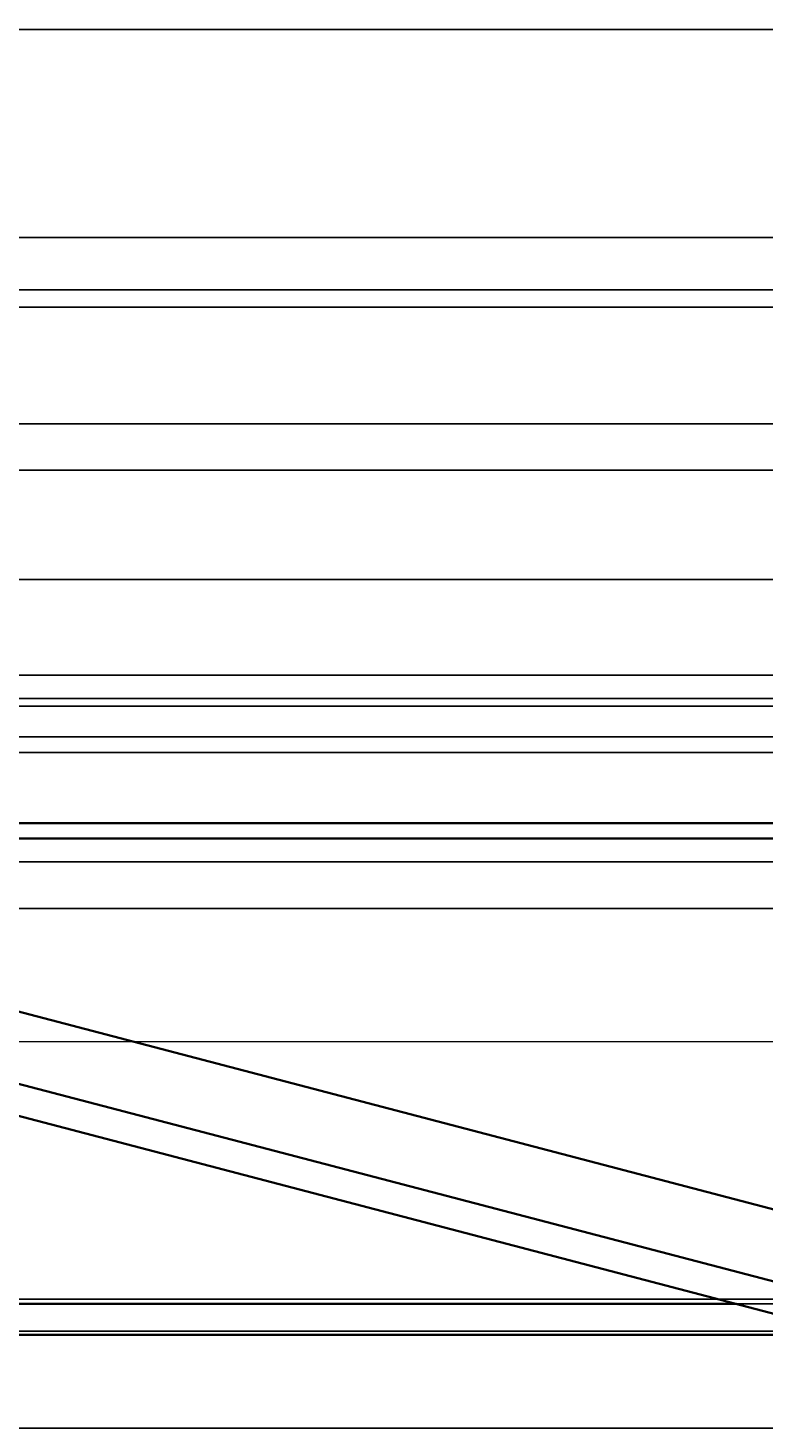
# Model space of a CAD drawing. Units: inches. Extents: x 2154 to 2740, y 571 to 1084.
# Tile 12 of 13: x 2485 to 2580, y 904 to 1084. Entities that reach past the tile are written whole.
import ezdxf

# ---------------------------------------------------------------- set-up
doc = ezdxf.new("R2010")
doc.units = ezdxf.units.IN
doc.layers.add('A-ANNO-DIMS', color=2, linetype='Continuous', lineweight=18)
doc.layers.add('A-ROOF', color=1, linetype='Continuous', lineweight=35)
doc.styles.get("Standard").update_dxf_attribs({"font": 'arial.ttf'})
doc.dimstyles.get("Standard").update_dxf_attribs({"dimtxt": 0.18, "dimasz": 0.18, "dimexe": 0.18, "dimexo": 0.0625, "dimgap": 0.09, "dimtad": 0, "dimtih": 1, "dimtoh": 1, "dimdec": 4, "dimzin": 0, "dimdsep": 46, "dimtxsty": 'Standard', "dimcen": 0.09, "dimadec": 0, "dimazin": 0, "dimtfac": 1, "dimtdec": 4, "dimtofl": 0, "dimtmove": 0, "dimatfit": 3, "dimfxl": 1, "dimtolj": 1, "dimtzin": 0, "dimarcsym": 0})

# ---------------------------------------------------------------- blocks, each defined once
blk = doc.blocks.new('*D7')
at = {"layer": 'A-ANNO-DIMS', "color": 0, "lineweight": -2, "transparency": 16777216}
for p, q in [((2181.21, 981.59), (2181.21, 1084.04)), ((2181.39, 1083.86), (2446.92, 1083.86)), ((2713.03, 1083.86), (2447.49, 1083.86)), ((2713.21, 981.59), (2713.21, 1084.04))]:
    blk.add_line(p, q, dxfattribs=at)
at = {"layer": 'A-ANNO-DIMS', "color": 0, "transparency": 16777216}
for points in [[(2181.39, 1083.89), (2181.39, 1083.83), (2181.21, 1083.86)], [(2713.03, 1083.89), (2713.03, 1083.83), (2713.21, 1083.86)]]:
    blk.add_solid(points, dxfattribs=at)
at = {"layer": 'Defpoints', "color": 0, "transparency": 16777216}
for p in [(2713.21, 1083.86), (2181.21, 981.53), (2713.21, 981.53)]:
    blk.add_point(p, dxfattribs=at)
at = {"layer": 'A-ANNO-DIMS', "color": 0, "transparency": 16777216, "insert": (2447.21, 1083.86), "char_height": 0.18, "attachment_point": 5}
blk.add_mtext('\\A1;532', dxfattribs=at)
blk = doc.blocks.new('*D8')
at = {"layer": 'A-ANNO-DIMS', "color": 0, "lineweight": -2, "transparency": 16777216}
for p, q in [((2284.21, 926.63), (2284.21, 953.59)), ((2284.39, 953.41), (2442.43, 953.37)), ((2601.03, 953.33), (2443, 953.37)), ((2601.21, 926.54), (2601.21, 953.51))]:
    blk.add_line(p, q, dxfattribs=at)
at = {"layer": 'A-ANNO-DIMS', "color": 0, "transparency": 16777216}
for points in [[(2284.39, 953.44), (2284.39, 953.38), (2284.21, 953.41)], [(2601.03, 953.36), (2601.03, 953.3), (2601.21, 953.33)]]:
    blk.add_solid(points, dxfattribs=at)
at = {"layer": 'Defpoints', "color": 0, "transparency": 16777216}
for p in [(2601.21, 953.33), (2284.21, 926.56), (2601.21, 926.48)]:
    blk.add_point(p, dxfattribs=at)
at = {"layer": 'A-ANNO-DIMS', "color": 0, "transparency": 16777216, "insert": (2442.71, 953.37), "char_height": 0.18, "attachment_point": 5}
blk.add_mtext('\\A1;317', dxfattribs=at)
blk = doc.blocks.new('*D13')
at = {"layer": 'A-ANNO-DIMS', "color": 0, "lineweight": -2, "transparency": 16777216}
for p, q in [((2447.27, 1057.01), (2740.24, 1057.01)), ((2740.06, 1056.83), (2740.06, 1019.45)), ((2740.06, 981.71), (2740.06, 1019.09)), ((2713.27, 981.53), (2740.24, 981.53))]:
    blk.add_line(p, q, dxfattribs=at)
at = {"layer": 'A-ANNO-DIMS', "color": 0, "transparency": 16777216}
for points in [[(2740.03, 1056.83), (2740.09, 1056.83), (2740.06, 1057.01)], [(2740.03, 981.71), (2740.09, 981.71), (2740.06, 981.53)]]:
    blk.add_solid(points, dxfattribs=at)
at = {"layer": 'Defpoints', "color": 0, "transparency": 16777216}
for p in [(2447.21, 1057.01), (2740.06, 1057.01), (2713.21, 981.53)]:
    blk.add_point(p, dxfattribs=at)
at = {"layer": 'A-ANNO-DIMS', "color": 0, "transparency": 16777216, "insert": (2740.06, 1019.27), "char_height": 0.18, "attachment_point": 5}
blk.add_mtext('\\A1;75.47', dxfattribs=at)
blk = doc.blocks.new('*D46')
at = {"layer": 'A-ANNO-DIMS', "color": 0, "lineweight": -2, "transparency": 16777216}
for p, q in [((2195.27, 915.53), (2740.24, 915.53)), ((2740.06, 915.35), (2740.06, 909.71)), ((2740.06, 903.71), (2740.06, 909.35)), ((2195.27, 903.53), (2740.24, 903.53))]:
    blk.add_line(p, q, dxfattribs=at)
at = {"layer": 'A-ANNO-DIMS', "color": 0, "transparency": 16777216}
for points in [[(2740.03, 915.35), (2740.09, 915.35), (2740.06, 915.53)], [(2740.03, 903.71), (2740.09, 903.71), (2740.06, 903.53)]]:
    blk.add_solid(points, dxfattribs=at)
at = {"layer": 'Defpoints', "color": 0, "transparency": 16777216}
for p in [(2195.21, 915.53), (2740.06, 915.53), (2195.21, 903.53)]:
    blk.add_point(p, dxfattribs=at)
at = {"layer": 'A-ANNO-DIMS', "color": 0, "transparency": 16777216, "insert": (2740.06, 909.53), "char_height": 0.18, "attachment_point": 5}
blk.add_mtext('\\A1;12', dxfattribs=at)
blk = doc.blocks.new('*D47')
at = {"layer": 'A-ANNO-DIMS', "color": 0, "lineweight": -2, "transparency": 16777216}
for p, q in [((2195.269199, 919.532069), (2740.236699, 919.532069)), ((2740.056699, 919.352069), (2740.056699, 917.712069)), ((2740.056699, 915.712069), (2740.056699, 917.352069)), ((2195.269199, 915.532069), (2740.236699, 915.532069))]:
    blk.add_line(p, q, dxfattribs=at)
at = {"layer": 'A-ANNO-DIMS', "color": 0, "transparency": 16777216}
for points in [[(2740.026699, 919.352069), (2740.086699, 919.352069), (2740.056699, 919.532069)], [(2740.026699, 915.712069), (2740.086699, 915.712069), (2740.056699, 915.532069)]]:
    blk.add_solid(points, dxfattribs=at)
at = {"layer": 'Defpoints', "color": 0, "transparency": 16777216}
for p in [(2195.206699, 919.532069), (2740.056699, 919.532069), (2195.206699, 915.532069)]:
    blk.add_point(p, dxfattribs=at)
at = {"layer": 'A-ANNO-DIMS', "color": 0, "transparency": 16777216, "insert": (2740.056699, 917.532069), "char_height": 0.18, "attachment_point": 5}
blk.add_mtext('\\A1;4', dxfattribs=at)
blk = doc.blocks.new('*D48')
at = {"layer": 'A-ANNO-DIMS', "color": 0, "lineweight": -2, "transparency": 16777216}
for p, q in [((2195.27, 979.53), (2740.24, 979.53)), ((2740.06, 979.35), (2740.06, 949.71)), ((2740.06, 919.71), (2740.06, 949.35)), ((2195.27, 919.53), (2740.24, 919.53))]:
    blk.add_line(p, q, dxfattribs=at)
at = {"layer": 'A-ANNO-DIMS', "color": 0, "transparency": 16777216}
for points in [[(2740.03, 979.35), (2740.09, 979.35), (2740.06, 979.53)], [(2740.03, 919.71), (2740.09, 919.71), (2740.06, 919.53)]]:
    blk.add_solid(points, dxfattribs=at)
at = {"layer": 'Defpoints', "color": 0, "transparency": 16777216}
for p in [(2195.21, 979.53), (2740.06, 979.53), (2195.21, 919.53)]:
    blk.add_point(p, dxfattribs=at)
at = {"layer": 'A-ANNO-DIMS', "color": 0, "transparency": 16777216, "insert": (2740.06, 949.53), "char_height": 0.18, "attachment_point": 5}
blk.add_mtext('\\A1;60', dxfattribs=at)
blk = doc.blocks.new('*D55')
at = {"layer": 'A-ANNO-DIMS', "color": 0, "lineweight": -2, "transparency": 16777216}
for p, q in [((2295.84, 920.15), (2740.24, 920.15)), ((2740.06, 919.97), (2740.06, 918.27)), ((2740.06, 916.21), (2740.06, 917.91)), ((2295.83, 916.03), (2740.24, 916.03))]:
    blk.add_line(p, q, dxfattribs=at)
at = {"layer": 'A-ANNO-DIMS', "color": 0, "transparency": 16777216}
for points in [[(2740.03, 919.97), (2740.09, 919.97), (2740.06, 920.15)], [(2740.03, 916.21), (2740.09, 916.21), (2740.06, 916.03)]]:
    blk.add_solid(points, dxfattribs=at)
at = {"layer": 'Defpoints', "color": 0, "transparency": 16777216}
for p in [(2295.77, 920.15), (2740.06, 920.15), (2295.77, 916.03)]:
    blk.add_point(p, dxfattribs=at)
at = {"layer": 'A-ANNO-DIMS', "color": 0, "transparency": 16777216, "insert": (2740.06, 918.09), "char_height": 0.18, "attachment_point": 5}
blk.add_mtext('\\A1;4.12', dxfattribs=at)
blk = doc.blocks.new('*D69')
at = {"layer": 'A-ANNO-DIMS', "color": 0, "lineweight": -2, "transparency": 16777216}
for p, q in [((2447.27, 1057.01), (2740.24, 1057.01)), ((2740.06, 1056.83), (2740.06, 1053.83)), ((2740.06, 1050.47), (2740.06, 1053.47)), ((2447.27, 1050.29), (2740.24, 1050.29))]:
    blk.add_line(p, q, dxfattribs=at)
at = {"layer": 'A-ANNO-DIMS', "color": 0, "transparency": 16777216}
for points in [[(2740.03, 1056.83), (2740.09, 1056.83), (2740.06, 1057.01)], [(2740.03, 1050.47), (2740.09, 1050.47), (2740.06, 1050.29)]]:
    blk.add_solid(points, dxfattribs=at)
at = {"layer": 'Defpoints', "color": 0, "transparency": 16777216}
for p in [(2447.21, 1057.01), (2740.06, 1057.01), (2447.21, 1050.29)]:
    blk.add_point(p, dxfattribs=at)
at = {"layer": 'A-ANNO-DIMS', "color": 0, "transparency": 16777216, "insert": (2740.06, 1053.65), "char_height": 0.18, "attachment_point": 5}
blk.add_mtext('\\A1;6.712', dxfattribs=at)
blk = doc.blocks.new('*D70')
at = {"layer": 'A-ANNO-DIMS', "color": 0, "lineweight": -2, "transparency": 16777216}
for p, q in [((2447.27, 1050.29), (2740.24, 1050.29)), ((2740.06, 1050.11), (2740.06, 1049.36)), ((2740.06, 1048.24), (2740.06, 1048.99)), ((2447.27, 1048.06), (2740.24, 1048.06))]:
    blk.add_line(p, q, dxfattribs=at)
at = {"layer": 'A-ANNO-DIMS', "color": 0, "transparency": 16777216}
for points in [[(2740.03, 1050.11), (2740.09, 1050.11), (2740.06, 1050.29)], [(2740.03, 1048.24), (2740.09, 1048.24), (2740.06, 1048.06)]]:
    blk.add_solid(points, dxfattribs=at)
at = {"layer": 'Defpoints', "color": 0, "transparency": 16777216}
for p in [(2447.21, 1050.29), (2740.06, 1050.29), (2447.21, 1048.06)]:
    blk.add_point(p, dxfattribs=at)
at = {"layer": 'A-ANNO-DIMS', "color": 0, "transparency": 16777216, "insert": (2740.06, 1049.17), "char_height": 0.18, "attachment_point": 5}
blk.add_mtext('\\A1;2.24', dxfattribs=at)
blk = doc.blocks.new('*D71')
at = {"layer": 'A-ANNO-DIMS', "color": 0, "lineweight": -2, "transparency": 16777216}
for p, q in [((2477.27, 1033.01), (2740.24, 1033.01)), ((2740.06, 1032.83), (2740.06, 1030.2)), ((2740.06, 1027.19), (2740.06, 1029.83)), ((2477.27, 1027.01), (2740.24, 1027.01))]:
    blk.add_line(p, q, dxfattribs=at)
at = {"layer": 'A-ANNO-DIMS', "color": 0, "transparency": 16777216}
for points in [[(2740.03, 1032.83), (2740.09, 1032.83), (2740.06, 1033.01)], [(2740.03, 1027.19), (2740.09, 1027.19), (2740.06, 1027.01)]]:
    blk.add_solid(points, dxfattribs=at)
at = {"layer": 'Defpoints', "color": 0, "transparency": 16777216}
for p in [(2477.21, 1033.01), (2740.06, 1033.01), (2477.21, 1027.01)]:
    blk.add_point(p, dxfattribs=at)
at = {"layer": 'A-ANNO-DIMS', "color": 0, "transparency": 16777216, "insert": (2740.06, 1030.01), "char_height": 0.18, "attachment_point": 5}
blk.add_mtext('\\A1;6', dxfattribs=at)
blk = doc.blocks.new('*D72')
at = {"layer": 'A-ANNO-DIMS', "color": 0, "lineweight": -2, "transparency": 16777216}
for p, q in [((2477.27, 1027.01), (2740.24, 1027.01)), ((2740.06, 1026.83), (2740.06, 1001.96)), ((2740.06, 976.71), (2740.06, 1001.59)), ((2477.27, 976.53), (2740.24, 976.53))]:
    blk.add_line(p, q, dxfattribs=at)
at = {"layer": 'A-ANNO-DIMS', "color": 0, "transparency": 16777216}
for points in [[(2740.03, 1026.83), (2740.09, 1026.83), (2740.06, 1027.01)], [(2740.03, 976.71), (2740.09, 976.71), (2740.06, 976.53)]]:
    blk.add_solid(points, dxfattribs=at)
at = {"layer": 'Defpoints', "color": 0, "transparency": 16777216}
for p in [(2477.21, 1027.01), (2740.06, 1027.01), (2477.21, 976.53)]:
    blk.add_point(p, dxfattribs=at)
at = {"layer": 'A-ANNO-DIMS', "color": 0, "transparency": 16777216, "insert": (2740.06, 1001.77), "char_height": 0.18, "attachment_point": 5}
blk.add_mtext('\\A1;50.48', dxfattribs=at)
blk = doc.blocks.new('*D73')
at = {"layer": 'A-ANNO-DIMS', "color": 0, "lineweight": -2, "transparency": 16777216}
for p, q in [((2477.27, 976.53), (2740.24, 976.53)), ((2740.06, 976.35), (2740.06, 973.71)), ((2740.06, 970.71), (2740.06, 973.35)), ((2477.27, 970.53), (2740.24, 970.53))]:
    blk.add_line(p, q, dxfattribs=at)
at = {"layer": 'A-ANNO-DIMS', "color": 0, "transparency": 16777216}
for points in [[(2740.03, 976.35), (2740.09, 976.35), (2740.06, 976.53)], [(2740.03, 970.71), (2740.09, 970.71), (2740.06, 970.53)]]:
    blk.add_solid(points, dxfattribs=at)
at = {"layer": 'Defpoints', "color": 0, "transparency": 16777216}
for p in [(2477.21, 976.53), (2740.06, 976.53), (2477.21, 970.53)]:
    blk.add_point(p, dxfattribs=at)
at = {"layer": 'A-ANNO-DIMS', "color": 0, "transparency": 16777216, "insert": (2740.06, 973.53), "char_height": 0.18, "attachment_point": 5}
blk.add_mtext('\\A1;6', dxfattribs=at)
blk = doc.blocks.new('*D78')
at = {"layer": 'A-ANNO-DIMS', "color": 0, "lineweight": -2, "transparency": 16777216}
for p, q in [((2459.95, 1012.91), (2740.24, 1012.91)), ((2740.06, 1012.73), (2740.06, 1001.95)), ((2740.06, 990.82), (2740.06, 1001.59)), ((2459.95, 990.64), (2740.24, 990.64))]:
    blk.add_line(p, q, dxfattribs=at)
at = {"layer": 'A-ANNO-DIMS', "color": 0, "transparency": 16777216}
for points in [[(2740.03, 1012.73), (2740.09, 1012.73), (2740.06, 1012.91)], [(2740.03, 990.82), (2740.09, 990.82), (2740.06, 990.64)]]:
    blk.add_solid(points, dxfattribs=at)
at = {"layer": 'Defpoints', "color": 0, "transparency": 16777216}
for p in [(2459.89, 1012.91), (2740.06, 1012.91), (2459.89, 990.64)]:
    blk.add_point(p, dxfattribs=at)
at = {"layer": 'A-ANNO-DIMS', "color": 0, "transparency": 16777216, "insert": (2740.06, 1001.77), "char_height": 0.18, "attachment_point": 5}
blk.add_mtext('\\A1;22.27', dxfattribs=at)
blk = doc.blocks.new('*D83')
at = {"layer": 'A-ANNO-DIMS', "color": 0, "lineweight": -2, "transparency": 16777216}
for p, q in [((2457.95, 996.6), (2740.24, 996.6)), ((2740.06, 996.42), (2740.06, 994.8)), ((2740.06, 992.82), (2740.06, 994.44)), ((2457.95, 992.64), (2740.24, 992.64))]:
    blk.add_line(p, q, dxfattribs=at)
at = {"layer": 'A-ANNO-DIMS', "color": 0, "transparency": 16777216}
for points in [[(2740.03, 996.42), (2740.09, 996.42), (2740.06, 996.6)], [(2740.03, 992.82), (2740.09, 992.82), (2740.06, 992.64)]]:
    blk.add_solid(points, dxfattribs=at)
at = {"layer": 'Defpoints', "color": 0, "transparency": 16777216}
for p in [(2457.89, 996.6), (2740.06, 996.6), (2457.89, 992.64)]:
    blk.add_point(p, dxfattribs=at)
at = {"layer": 'A-ANNO-DIMS', "color": 0, "transparency": 16777216, "insert": (2740.06, 994.62), "char_height": 0.18, "attachment_point": 5}
blk.add_mtext('\\A1;3.964', dxfattribs=at)
blk = doc.blocks.new('*D84')
at = {"layer": 'A-ANNO-DIMS', "color": 0, "lineweight": -2, "transparency": 16777216}
for p, q in [((2457.95, 997.6), (2740.24, 997.6)), ((2457.95, 996.6), (2740.24, 996.6)), ((2740.06, 997.42), (2740.06, 997.28)), ((2740.06, 996.78), (2740.06, 996.92))]:
    blk.add_line(p, q, dxfattribs=at)
at = {"layer": 'A-ANNO-DIMS', "color": 0, "transparency": 16777216}
for points in [[(2740.03, 997.42), (2740.09, 997.42), (2740.06, 997.6)], [(2740.03, 996.78), (2740.09, 996.78), (2740.06, 996.6)]]:
    blk.add_solid(points, dxfattribs=at)
at = {"layer": 'Defpoints', "color": 0, "transparency": 16777216}
for p in [(2457.89, 997.6), (2457.89, 996.6), (2740.06, 997.6)]:
    blk.add_point(p, dxfattribs=at)
at = {"layer": 'A-ANNO-DIMS', "color": 0, "transparency": 16777216, "insert": (2740.06, 997.1), "char_height": 0.18, "attachment_point": 5}
blk.add_mtext('\\A1;1', dxfattribs=at)
blk = doc.blocks.new('*D85')
at = {"layer": 'A-ANNO-DIMS', "color": 0, "lineweight": -2, "transparency": 16777216}
for p, q in [((2457.95, 1000.6), (2740.24, 1000.6)), ((2740.06, 1000.42), (2740.06, 999.28)), ((2740.06, 997.78), (2740.06, 998.92)), ((2457.95, 997.6), (2740.24, 997.6))]:
    blk.add_line(p, q, dxfattribs=at)
at = {"layer": 'A-ANNO-DIMS', "color": 0, "transparency": 16777216}
for points in [[(2740.03, 1000.42), (2740.09, 1000.42), (2740.06, 1000.6)], [(2740.03, 997.78), (2740.09, 997.78), (2740.06, 997.6)]]:
    blk.add_solid(points, dxfattribs=at)
at = {"layer": 'Defpoints', "color": 0, "transparency": 16777216}
for p in [(2457.89, 1000.6), (2740.06, 1000.6), (2457.89, 997.6)]:
    blk.add_point(p, dxfattribs=at)
at = {"layer": 'A-ANNO-DIMS', "color": 0, "transparency": 16777216, "insert": (2740.06, 999.1), "char_height": 0.18, "attachment_point": 5}
blk.add_mtext('\\A1;3', dxfattribs=at)

msp = doc.modelspace()

# ---------------------------------------------------------------- linework, layer by layer
at = {"layer": 'A-ROOF'}
for p, q in [((2477.2067, 981.5321), (2713.2067, 981.5321)), ((2477.2067, 979.5321), (2711.2067, 979.5321)), ((2447.273, 966.8186), (2601.2067, 926.4774)), ((2447.2067, 957.5321), (2590.2325, 920.0494)), ((2447.1772, 953.4047), (2590.1732, 915.9299)), ((2309.9659, 919.5321), (2576.4281, 919.5321)), ((2195.2067, 915.5321), (2699.2067, 915.5321))]:
    msp.add_line(p, q, dxfattribs=at)

# ---------------------------------------------------------------- dimensions: what is measured, and where the dimension line sits
at = {"layer": 'A-ANNO-DIMS'}
dim = msp.add_linear_dim(base=(2713.2067, 1083.8553), p1=(2181.2067, 981.5321), p2=(2713.2067, 981.5321), dimstyle='Standard', override={"dimdec": 0, "dimlfac": 1, "dimrnd": 0, "dimzin": 0, "dimdsep": 46, "dimlunit": 2}, dxfattribs=at)
dim.commit()
dim.dimension.update_dxf_attribs({"geometry": '*D7', "text_midpoint": (2447.2067, 1083.8553)})
for base, p1, p2, angle, override, picture, middle in [((2740.0567, 1057.0053), (2713.2067, 981.5321), (2447.2067, 1057.0053), 90, {"dimdec": 2, "dimlfac": 1, "dimrnd": 0, "dimzin": 0, "dimdsep": 46, "dimlunit": 2}, '*D13', (2740.0567, 1019.2687)), ((2740.0567, 1057.0053), (2447.2067, 1050.2934), (2447.2067, 1057.0053), 90, {"dimdec": 3, "dimlfac": 1, "dimrnd": 0, "dimzin": 0, "dimdsep": 46, "dimlunit": 2}, '*D69', (2740.0567, 1053.6493)), ((2740.0567, 1050.2934), (2447.2067, 1048.0561), (2447.2067, 1050.2934), 90, {"dimdec": 2, "dimlfac": 1, "dimrnd": 0, "dimzin": 0, "dimdsep": 46, "dimlunit": 2}, '*D70', (2740.0567, 1049.1747)), ((2740.0567, 1033.0148), (2477.2067, 1027.0148), (2477.2067, 1033.0148), 90, {"dimdec": 0, "dimlfac": 1, "dimrnd": 0, "dimzin": 0, "dimdsep": 46, "dimlunit": 2}, '*D71', (2740.0567, 1030.0148)), ((2740.0567, 1027.0148), (2477.2067, 976.5321), (2477.2067, 1027.0148), 90, {"dimdec": 2, "dimlfac": 1, "dimrnd": 0, "dimzin": 0, "dimdsep": 46, "dimlunit": 2}, '*D72', (2740.0567, 1001.7734)), ((2740.0567, 1012.9076), (2459.8896, 990.6361), (2459.8896, 1012.9076), 90, {"dimdec": 2, "dimlfac": 1, "dimrnd": 0, "dimzin": 0, "dimdsep": 46, "dimlunit": 2}, '*D78', (2740.0567, 1001.7719)), ((2740.0567, 1000.5998), (2457.8896, 997.5998), (2457.8896, 1000.5998), 90, {"dimdec": 0, "dimlfac": 1, "dimrnd": 0, "dimzin": 0, "dimdsep": 46, "dimlunit": 2}, '*D85', (2740.0567, 999.0998)), ((2740.0567, 997.5998), (2457.8896, 996.5998), (2457.8896, 997.5998), 90, {"dimdec": 0, "dimlfac": 1, "dimrnd": 0, "dimzin": 0, "dimdsep": 46, "dimlunit": 2}, '*D84', (2740.0567, 997.0998)), ((2740.0567, 996.5998), (2457.8896, 992.6361), (2457.8896, 996.5998), 90, {"dimdec": 3, "dimlfac": 1, "dimrnd": 0, "dimzin": 0, "dimdsep": 46, "dimlunit": 2}, '*D83', (2740.0567, 994.618)), ((2740.0567, 979.5321), (2195.2067, 919.5321), (2195.2067, 979.5321), 90, {"dimdec": 0, "dimlfac": 1, "dimrnd": 0, "dimzin": 0, "dimdsep": 46, "dimlunit": 2}, '*D48', (2740.0567, 949.5321)), ((2740.0567, 976.5321), (2477.2067, 970.5321), (2477.2067, 976.5321), 90, {"dimdec": 0, "dimlfac": 1, "dimrnd": 0, "dimzin": 0, "dimdsep": 46, "dimlunit": 2}, '*D73', (2740.0567, 973.5321)), ((2601.214, 953.3274), (2284.2067, 926.5633), (2601.2067, 926.4774), 359.984471, {"dimdec": 0, "dimlfac": 1, "dimrnd": 0, "dimzin": 0, "dimdsep": 46, "dimlunit": 2}, '*D8', (2442.714, 953.3703)), ((2740.0567, 919.5321), (2195.2067, 915.5321), (2195.2067, 919.5321), 90, {"dimdec": 0, "dimlfac": 1, "dimrnd": 0, "dimzin": 0, "dimdsep": 46, "dimlunit": 2}, '*D47', (2740.0567, 917.5321)), ((2740.0567, 920.1485), (2295.7714, 916.028), (2295.7731, 920.1485), 90, {"dimdec": 2, "dimlfac": 1, "dimrnd": 0, "dimzin": 0, "dimdsep": 46, "dimlunit": 2}, '*D55', (2740.0567, 918.0882)), ((2740.0567, 915.5321), (2195.2067, 903.5321), (2195.2067, 915.5321), 90, {"dimdec": 0, "dimlfac": 1, "dimrnd": 0, "dimzin": 0, "dimdsep": 46, "dimlunit": 2}, '*D46', (2740.0567, 909.5321))]:
    dim = msp.add_linear_dim(base=base, p1=p1, p2=p2, angle=angle, dimstyle='Standard', override=override, dxfattribs=at)
    dim.commit()
    dim.dimension.update_dxf_attribs({"geometry": picture, "text_midpoint": middle})

doc.saveas('drawing.dxf')
